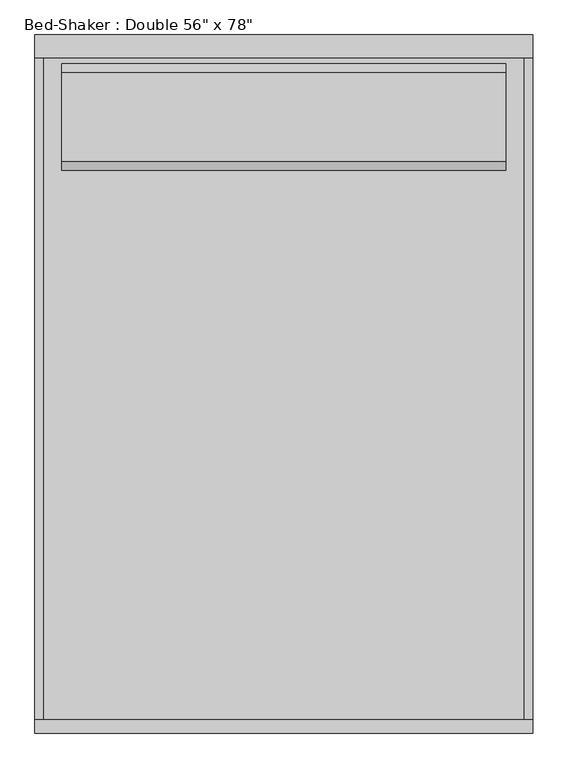
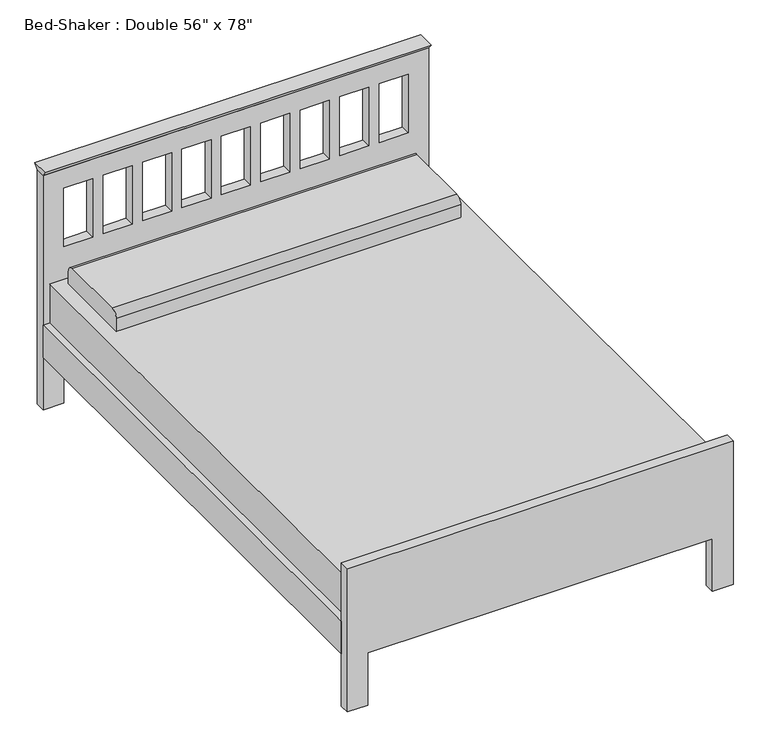
"""IFC4 building model written with IfcOpenShell, lengths in millimetres: furniture geometry."""

from ifc_helpers import new_model, si_unit, point, frame, frame_2d, origin, place, context, project, spatial, polyline, circle_curve, trimmed, segment, composite_curve, outline, extrude, source, transform, mapped, element, save


def furniture_096e7f55(model_context):
    return source(origin(), model_context, "Body", "SweptSolid", [
        extrude(outline(polyline([(-38.1, 914.4), (-51.9545455, 933.45), (13.8545455, 933.45), (0.0, 914.4), (-38.1, 914.4)])), frame((-730.0365546, 0.0, 0.0), z_axis=(1.0, 0.0, 0.0), x_axis=(0.0, 1.0, 0.0)), (0.0, 0.0, 1.0), 1422.4533613),
        extrude(outline(composite_curve([segment(polyline([(-373.2486637, 482.6), (-373.2486637, 533.4)]), True, "CONTINUOUS"), segment(trimmed(circle_curve(frame_2d((-347.8486637, 533.4)), 25.4), [point((-373.2486637, 533.4))], [point((-347.8486637, 558.8))], False, "CARTESIAN"), True, "CONTINUOUS"), segment(polyline([(-347.8486637, 558.8), (-93.8486637, 558.8)]), True, "CONTINUOUS"), segment(trimmed(circle_curve(frame_2d((-93.8486637, 533.4)), 25.4), [point((-93.8486637, 558.8))], [point((-68.4486637, 533.4))], False, "CARTESIAN"), True, "CONTINUOUS"), segment(polyline([(-68.4486637, 533.4), (-68.4486637, 482.6), (-373.2486637, 482.6)]), True, "CONTINUOUS")], self_intersect=False)), frame((-654.05, 0.0, 0.0), z_axis=(1.0, 0.0, 0.0), x_axis=(0.0, 1.0, 0.0)), (0.0, 0.0, 1.0), 1270.0),
        extrude(outline(polyline([(666.75, -38.1), (666.75, -1943.1), (-704.85, -1943.1), (-704.85, -38.1), (666.75, -38.1)])), frame((0.0, 0.0, 228.6), z_axis=(0.0, 0.0, 1.0), x_axis=(1.0, 0.0, 0.0)), (0.0, 0.0, 1.0), 254.0),
        extrude(outline(polyline([(666.75, -1943.1), (666.75, -38.1), (692.15, -38.1), (692.15, -1943.1), (666.75, -1943.1)])), frame((0.0, 0.0, 203.0994861), z_axis=(0.0, 0.0, 1.0), x_axis=(1.0, 0.0, 0.0)), (0.0, 0.0, 1.0), 127.0),
        extrude(outline(polyline([(-730.25, -1943.1), (-730.25, -38.1), (-704.85, -38.1), (-704.85, -1943.1), (-730.25, -1943.1)])), frame((0.0, 0.0, 203.5755296), z_axis=(0.0, 0.0, 1.0), x_axis=(1.0, 0.0, 0.0)), (0.0, 0.0, 1.0), 127.0),
        extrude(outline(polyline([(0.0, -654.05), (203.2, -654.05), (203.2, 615.95), (0.0, 615.95), (0.0, 692.15), (558.8, 692.15), (558.8, -730.25), (0.0, -730.25), (0.0, -654.05)])), frame((0.0, -1981.2, 0.0), z_axis=(0.0, 1.0, 0.0), x_axis=(0.0, 0.0, 1.0)), (0.0, 0.0, 1.0), 38.1),
        extrude(outline(polyline([(914.4, 692.4168067), (914.4, -730.0365546), (0.0, -730.0365546), (0.0, -654.05), (203.2, -654.05), (203.2, 615.95), (0.0, 615.95), (0.0, 692.4168067), (914.4, 692.4168067)]), holes=[polyline([(838.2, -546.8055556), (609.6, -546.8055556), (609.6, -654.05), (838.2, -654.05), (838.2, -546.8055556)]), polyline([(838.2, -401.4611111), (609.6, -401.4611111), (609.6, -508.7055556), (838.2, -508.7055556), (838.2, -401.4611111)]), polyline([(838.2, -256.1166667), (609.6, -256.1166667), (609.6, -363.3611111), (838.2, -363.3611111), (838.2, -256.1166667)]), polyline([(838.2, -110.7722222), (609.6, -110.7722222), (609.6, -218.0166667), (838.2, -218.0166667), (838.2, -110.7722222)]), polyline([(838.2, 179.9166667), (609.6, 179.9166667), (609.6, 72.6722222), (838.2, 72.6722222), (838.2, 179.9166667)]), polyline([(838.2, 325.2611111), (609.6, 325.2611111), (609.6, 218.0166667), (838.2, 218.0166667), (838.2, 325.2611111)]), polyline([(838.2, 470.6055556), (609.6, 470.6055556), (609.6, 363.3611111), (838.2, 363.3611111), (838.2, 470.6055556)]), polyline([(838.2, 615.95), (609.6, 615.95), (609.6, 508.7055556), (838.2, 508.7055556), (838.2, 615.95)]), polyline([(838.2, 34.5722222), (609.6, 34.5722222), (609.6, -72.6722222), (838.2, -72.6722222), (838.2, 34.5722222)])]), frame((0.0, -38.1, 0.0), z_axis=(0.0, 1.0, 0.0), x_axis=(0.0, 0.0, 1.0)), (0.0, 0.0, 1.0), 38.1),
    ])


if __name__ == "__main__":
    model = new_model("IFC4")
    model_context = context("Model", 3, world=origin())
    ifc_project = project(units=[si_unit("LENGTHUNIT", "METRE", prefix="MILLI")], contexts=[model_context])
    site = spatial("IfcSite", under=ifc_project)
    building = spatial("IfcBuilding", under=site)
    placement = place(None, origin())
    furniture_shape = furniture_096e7f55(model_context)
    element("IfcFurniture", 1, ObjectType="Bed-Shaker : Double 56\" x 78\"", at=placement, inside=building, context=model_context, shape_type="MappedRepresentation", body=[
        mapped(furniture_shape, transform((0.0, 0.0, 0.0), x_axis=(1.0, 0.0, 0.0), y_axis=(0.0, 1.0, 0.0), z_axis=(0.0, 0.0, 1.0))),
    ])
    save(model, "model.ifc")

# Revit data of these elements
# Type "Bed-Shaker : Double 56\" x 78\""
#   Assembly Code = "E2020200"
#   Length = 6' - 6"
#   Width = 4' - 8"
#   Frame Material = Birch
#   Mattress Material = Linen, White
#   Default Elevation = 0
# Element 1 (IfcFurniture, "Bed-Shaker : Double 56\" x 78\"")
#   Materials on its faces: "Birch", "Linen, White"
# Materials
#   "Birch": class "Wood", colour RGB 224 178 126, transparency 0, Description = "Betula Alleghaniensis", Cost = 0
#   "Linen, White": class "Textile", colour RGB 247 247 239, transparency 0, Description = "Linen, white", Cost = 0
